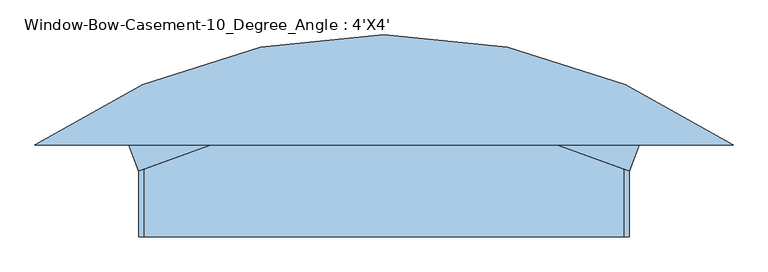
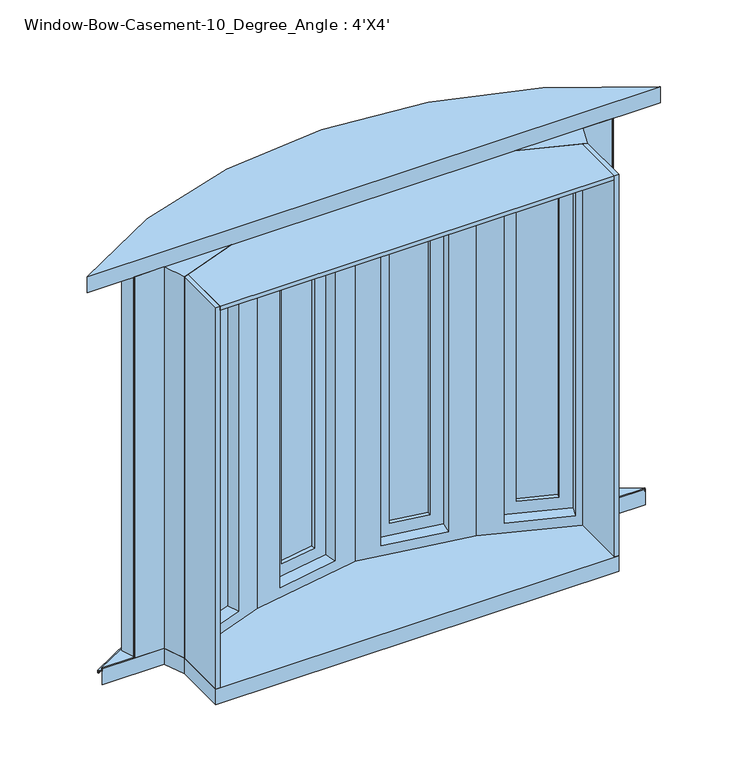
"""IFC4 building model written with IfcOpenShell, lengths in millimetres: window geometry, Window-Bow-Casement-10_Degree_Angle : 4'X4'."""

from ifc_helpers import new_model, si_unit, point, frame, frame_2d, origin, place, context, project, spatial, polyline, circle_curve, trimmed, segment, composite_curve, outline, extrude, faceted_brep, source, transform, mapped, element, save
from ifc_brep_helpers import plane_surface, cylinder_surface, revolved_surface, advanced_brep


def window_bow_casement_10_degree_angle_4_x4_fc1e5cf1(model_context):
    return source(origin(), model_context, "Body", "SolidModel", [
        advanced_brep(
        [(-820.9076978, 114.3, 663.1486341), (-820.9076978, 114.3, 660.4), (-728.4786409, 114.3, 660.4), (-728.4786409, 114.3, 663.1486341), (820.9076978, 114.3, 660.4), (820.9076978, 114.3, 663.1486341), (728.4786409, 114.3, 663.1486341), (728.4786409, 114.3, 660.4), (-820.9076978, 114.3, 653.0697935), (-821.7069058, 115.4458078, 663.1486341), (-821.7069058, 115.4458078, 654.4483503), (-828.9724329, 125.8622427, 652.2089977), (-828.9724329, 125.8622427, 643.2668038), (-826.7055885, 122.6123151, 643.2668038), (-826.7055885, 122.6123151, 644.7270038), (-828.0569765, 124.549772, 644.7270038), (-828.0569765, 124.549772, 650.8662705), (820.9076978, 114.3, 653.0697935), (828.0569765, 124.549772, 650.8662705), (828.0569765, 124.549772, 644.7270038), (826.7055885, 122.6123151, 644.7270038), (826.7055885, 122.6123151, 643.2668038), (828.9724329, 125.8622427, 643.2668038), (828.9724329, 125.8622427, 652.2089977), (821.7069058, 115.4458078, 654.4483503), (821.7069058, 115.4458078, 663.1486341)],
        [
            (0, 1),
            (1, 2),
            (2, 3),
            (3, 0),
            (4, 5),
            (5, 6),
            (6, 7),
            (7, 4),
            (8, 1),
            (0, 9),
            (9, 10),
            (10, 11),
            (11, 12),
            (12, 13),
            (13, 14),
            (14, 15),
            (15, 16),
            (16, 8),
            (17, 18),
            (18, 19),
            (19, 20),
            (20, 21),
            (21, 22),
            (22, 23),
            (23, 24),
            (24, 25),
            (25, 5),
            (4, 17),
            (8, 17, circle_curve(frame((0.0, -1062.6182794, 653.0697935), z_axis=(0.0, 0.0, -1.0), x_axis=(-0.5720887452257101, 0.8201917261141279, 0.0)), 1434.9306899)),
            (4, 1, circle_curve(frame((0.0, -1062.6182794, 660.4), z_axis=(0.0, 0.0, 1.0), x_axis=(-0.5720887452257101, 0.8201917261141279, 0.0)), 1434.9306899)),
            (7, 2, circle_curve(frame((0.0, -1062.6182794, 660.4), z_axis=(0.0, 0.0, 1.0), x_axis=(-0.5720887452257101, 0.8201917261141279, 0.0)), 1384.1306899)),
            (6, 3, circle_curve(frame((0.0, -1062.6182794, 663.1486341), z_axis=(0.0, 0.0, 1.0), x_axis=(-0.5720887452257101, 0.8201917261141279, 0.0)), 1384.1306899)),
            (25, 9, circle_curve(frame((0.0, -1062.6182794, 663.1486341), z_axis=(0.0, 0.0, 1.0), x_axis=(-0.5720887452257101, 0.8201917261141279, 0.0)), 1436.3276898)),
            (24, 10, circle_curve(frame((0.0, -1062.6182794, 654.4483503), z_axis=(0.0, 0.0, 1.0), x_axis=(-0.5720887452257101, 0.8201917261141279, 0.0)), 1436.3276898)),
            (23, 11, circle_curve(frame((0.0, -1062.6182794, 652.2089977), z_axis=(0.0, 0.0, 1.0), x_axis=(-0.5720887452257101, 0.8201917261141279, 0.0)), 1449.0276898)),
            (22, 12, circle_curve(frame((0.0, -1062.6182794, 643.2668038), z_axis=(0.0, 0.0, 1.0), x_axis=(-0.5720887452257101, 0.8201917261141279, 0.0)), 1449.0276898)),
            (21, 13, circle_curve(frame((0.0, -1062.6182794, 643.2668038), z_axis=(0.0, 0.0, 1.0), x_axis=(-0.5720887452257101, 0.8201917261141279, 0.0)), 1445.0652899)),
            (20, 14, circle_curve(frame((0.0, -1062.6182794, 644.7270038), z_axis=(0.0, 0.0, 1.0), x_axis=(-0.5720887452257101, 0.8201917261141279, 0.0)), 1445.0652899)),
            (19, 15, circle_curve(frame((0.0, -1062.6182794, 644.7270038), z_axis=(0.0, 0.0, 1.0), x_axis=(-0.5720887452257101, 0.8201917261141279, 0.0)), 1447.4274899)),
            (18, 16, circle_curve(frame((0.0, -1062.6182794, 650.8662705), z_axis=(0.0, 0.0, 1.0), x_axis=(-0.5720887452257101, 0.8201917261141279, 0.0)), 1447.4274899)),
        ],
        [
            plane_surface(frame((903.8545728, 114.3, 1270.0), z_axis=(0.0, -1.0, 0.0), x_axis=(0.0, 0.0, -1.0))),
            plane_surface(frame((-820.9076978, 114.3, 660.4), z_axis=(-0.8201917261141279, -0.5720887452257101, 0.0), x_axis=(0.0, 0.0, 1.0))),
            plane_surface(frame((820.9076978, 114.3, 660.4), z_axis=(0.8201917261141279, -0.5720887452257102, 0.0), x_axis=(0.0, 0.0, 1.0))),
            revolved_surface(polyline([(-820.9076978707535, 114.30000000321752, 653.0697935), (-820.9076978707535, 114.30000000321752, 660.4)]), (0.0, -1062.6182794, 660.4), (0.0, 0.0, -1.0)),
            plane_surface(frame((0.0, -1062.6182794, 660.4), z_axis=(0.0, 0.0, -1.0), x_axis=(-0.5720887452257101, 0.8201917261141279, 0.0))),
            revolved_surface(polyline([(-791.8455896132875, 72.63426031661993, 660.4), (-791.8455896132875, 72.63426031661993, 663.1486341)]), (0.0, -1062.6182794, 660.4), (0.0, 0.0, -1.0)),
            plane_surface(frame((0.0, -1062.6182794, 663.1486341), z_axis=(0.0, 0.0, 1.0), x_axis=(-0.5720887452257101, 0.8201917261141279, 0.0))),
            cylinder_surface(frame((0.0, -1062.6182794, 660.4), z_axis=(0.0, 0.0, -1.0), x_axis=(-0.5720887452257101, 0.8201917261141279, 0.0)), 1436.3276898),
            revolved_surface(polyline([(-821.7069058, 115.4458078, 654.4483503), (-828.9724329, 125.8622427, 652.2089977)]), (0.0, -1062.6182794, 660.4), (0.0, 0.0, -1.0)),
            cylinder_surface(frame((0.0, -1062.6182794, 660.4), z_axis=(0.0, 0.0, -1.0), x_axis=(-0.5720887452257101, 0.8201917261141279, 0.0)), 1449.0276898),
            plane_surface(frame((0.0, -1062.6182794, 643.2668038), z_axis=(0.0, 0.0, -1.0), x_axis=(-0.5720887452257101, 0.8201917261141279, 0.0))),
            revolved_surface(polyline([(-826.7055884681179, 122.61231507069374, 643.2668038), (-826.7055884681179, 122.61231507069374, 644.7270038)]), (0.0, -1062.6182794, 660.4), (0.0, 0.0, -1.0)),
            plane_surface(frame((0.0, -1062.6182794, 644.7270038), z_axis=(0.0, 0.0, 1.0), x_axis=(-0.5720887452257101, 0.8201917261141279, 0.0))),
            revolved_surface(polyline([(-828.0569765020902, 124.54977196612049, 644.7270038), (-828.0569765020902, 124.54977196612049, 650.8662705)]), (0.0, -1062.6182794, 660.4), (0.0, 0.0, -1.0)),
            revolved_surface(polyline([(-828.0569765, 124.549772, 650.8662705), (-820.9076978, 114.3, 653.0697935)]), (0.0, -1062.6182794, 660.4), (0.0, 0.0, -1.0)),
        ],
        [
            (0, [[1, 2, 3, 4]]),
            (0, [[5, 6, 7, 8]]),
            (1, [[9, -1, 10, 11, 12, 13, 14, 15, 16, 17, 18]]),
            (2, [[19, 20, 21, 22, 23, 24, 25, 26, 27, -5, 28]]),
            (3, [[-9, 29, -28, 30]]),
            (4, [[-30, -8, 31, -2]]),
            (5, [[-31, -7, 32, -3]]),
            (6, [[33, -10, -4, -32, -6, -27]]),
            (7, [[-11, -33, -26, 34]]),
            (8, [[-12, -34, -25, 35]]),
            (9, [[-13, -35, -24, 36]]),
            (10, [[-14, -36, -23, 37]]),
            (11, [[-15, -37, -22, 38]]),
            (12, [[-16, -38, -21, 39]]),
            (13, [[-17, -39, -20, 40]]),
            (14, [[-18, -40, -19, -29]]),
        ],
    ),
        extrude(outline(polyline([(-692.8458946, 125.1591396), (-722.6811353, 114.3), (-737.8839307, 156.069337), (-708.04869, 166.9284765), (-692.8458946, 125.1591396)])), frame((0.0, 0.0, 663.1486341), z_axis=(0.0, 0.0, 1.0), x_axis=(1.0, 0.0, 0.0)), (0.0, 0.0, 1.0), 1216.4513659),
        extrude(outline(polyline([(692.8458946, 125.1591396), (708.04869, 166.9284765), (737.8839307, 156.069337), (722.6811353, 114.3), (692.8458946, 125.1591396)])), frame((0.0, 0.0, 663.1486341), z_axis=(0.0, 0.0, 1.0), x_axis=(1.0, 0.0, 0.0)), (0.0, 0.0, 1.0), 1216.4513659),
        faceted_brep([(0.0, 208.5319163, 1879.6), (330.4505105, 150.2645755, 1879.6), (356.846972, 248.7775109, 1879.6), (0.0, 311.6992601, 1879.6), (280.5494558, 197.7512317, 1866.9), (57.0219627, 237.1651597, 1866.9), (68.048622, 299.700452, 1866.9), (291.5761151, 260.2865241, 1866.9), (255.1728726, 163.5380541, 1847.85), (69.1665548, 196.3359865, 1847.85), (75.7825504, 233.8571619, 1847.85), (261.7888681, 201.0592295, 1847.85), (57.0219627, 237.1651597, 673.1), (68.048622, 299.700452, 673.1), (69.1665548, 196.3359865, 692.15), (75.7825504, 233.8571619, 692.15), (0.0, 311.6992601, 660.4), (356.846972, 248.7775109, 660.4), (330.4505105, 150.2645755, 660.4), (0.0, 208.5319163, 660.4), (280.5494558, 197.7512317, 673.1), (291.5761151, 260.2865241, 673.1), (255.1728726, 163.5380541, 692.15), (261.7888681, 201.0592295, 692.15)], [[[0, 1, 2, 3]], [[4, 5, 6, 7]], [[8, 9, 10, 11]], [[5, 12, 13, 6]], [[9, 14, 15, 10]], [[16, 17, 18, 19]], [[12, 20, 21, 13]], [[14, 22, 23, 15]], [[2, 17, 16, 3], [6, 13, 21, 7]], [[7, 21, 20, 4]], [[4, 20, 12, 5], [10, 15, 23, 11]], [[11, 23, 22, 8]], [[18, 1, 0, 19], [8, 22, 14, 9]], [[3, 16, 19, 0]], [[1, 18, 17, 2]]]),
        extrude(outline(polyline([(229.7810224, 238.9428712), (228.6783565, 232.689342), (117.7143895, 252.2552833), (118.8170554, 258.5088125), (229.7810224, 238.9428712)])), frame((0.0, 0.0, 730.25), z_axis=(0.0, 0.0, 1.0), x_axis=(1.0, 0.0, 0.0)), (0.0, 0.0, 1.0), 1079.5),
        extrude(outline(polyline([(227.5756905, 226.4358128), (226.4730246, 220.1822836), (115.5090576, 239.7482248), (116.6117235, 246.0017541), (227.5756905, 226.4358128)])), frame((0.0, 0.0, 730.25), z_axis=(0.0, 0.0, 1.0), x_axis=(1.0, 0.0, 0.0)), (0.0, 0.0, 1.0), 1079.5),
        extrude(outline(polyline([(1136.65, 57.1499999), (1136.65, -169.8257651), (-57.15, -169.8257651), (-57.15, 57.1499999), (1136.65, 57.1499999)]), holes=[polyline([(1079.5, -112.6757651), (1079.5, 0.0), (0.0, 0.0), (0.0, -112.6757651), (1079.5, -112.6757651)])]), frame((224.2676928, 207.6752251, 730.25), z_axis=(0.17364817766693014, 0.9848077530122081, 0.0), x_axis=(0.0, 0.0, 1.0)), (0.0, 0.0, 1.0), 44.45),
        faceted_brep([(0.0, 208.5319163, 1879.6), (0.0, 311.6992601, 1879.6), (-356.846972, 248.7775109, 1879.6), (-330.4505105, 150.2645755, 1879.6), (-280.5494558, 197.7512317, 1866.9), (-291.5761151, 260.2865241, 1866.9), (-68.048622, 299.700452, 1866.9), (-57.0219627, 237.1651597, 1866.9), (-255.1728726, 163.5380541, 1847.85), (-261.7888681, 201.0592295, 1847.85), (-75.7825504, 233.8571619, 1847.85), (-69.1665548, 196.3359865, 1847.85), (-68.048622, 299.700452, 673.1), (-57.0219627, 237.1651597, 673.1), (-75.7825504, 233.8571619, 692.15), (-69.1665548, 196.3359865, 692.15), (0.0, 311.6992601, 660.4), (0.0, 208.5319163, 660.4), (-330.4505105, 150.2645755, 660.4), (-356.846972, 248.7775109, 660.4), (-291.5761151, 260.2865241, 673.1), (-280.5494558, 197.7512317, 673.1), (-261.7888681, 201.0592295, 692.15), (-255.1728726, 163.5380541, 692.15)], [[[0, 1, 2, 3]], [[4, 5, 6, 7]], [[8, 9, 10, 11]], [[7, 6, 12, 13]], [[11, 10, 14, 15]], [[16, 17, 18, 19]], [[13, 12, 20, 21]], [[15, 14, 22, 23]], [[2, 1, 16, 19], [6, 5, 20, 12]], [[5, 4, 21, 20]], [[4, 7, 13, 21], [10, 9, 22, 14]], [[9, 8, 23, 22]], [[18, 17, 0, 3], [8, 11, 15, 23]], [[1, 0, 17, 16]], [[3, 2, 19, 18]]]),
        extrude(outline(polyline([(-229.7810224, 238.9428712), (-118.8170554, 258.5088125), (-117.7143895, 252.2552833), (-228.6783565, 232.689342), (-229.7810224, 238.9428712)])), frame((0.0, 0.0, 730.25), z_axis=(0.0, 0.0, 1.0), x_axis=(1.0, 0.0, 0.0)), (0.0, 0.0, 1.0), 1079.5),
        extrude(outline(polyline([(-227.5756905, 226.4358128), (-116.6117235, 246.0017541), (-115.5090576, 239.7482248), (-226.4730246, 220.1822836), (-227.5756905, 226.4358128)])), frame((0.0, 0.0, 730.25), z_axis=(0.0, 0.0, 1.0), x_axis=(1.0, 0.0, 0.0)), (0.0, 0.0, 1.0), 1079.5),
        extrude(outline(polyline([(1136.65, -57.1499999), (-57.15, -57.1499999), (-57.15, 169.8257651), (1136.65, 169.8257651), (1136.65, -57.1499999)]), holes=[polyline([(1079.5, 112.6757651), (0.0, 112.6757651), (0.0, 0.0), (1079.5, 0.0), (1079.5, 112.6757651)])]), frame((-224.2676928, 207.6752251, 730.25), z_axis=(-0.17364817766693014, 0.9848077530122081, 0.0), x_axis=(0.0, 0.0, 1.0)), (0.0, 0.0, 1.0), 44.45),
        faceted_brep([(330.4505105, 150.2645755, 1879.6), (609.6, 48.6624704, 1879.6), (633.490107, 114.3, 1879.6), (726.3208967, 114.3, 1879.6), (356.846972, 248.7775109, 1879.6), (610.6968712, 88.8084151, 1866.9), (397.4094197, 166.4386988, 1866.9), (419.1276988, 226.1091802, 1866.9), (632.4151503, 148.4788965, 1866.9), (579.7647593, 59.52161, 1847.85), (402.2795966, 124.1209262, 1847.85), (415.3105641, 159.9232151, 1847.85), (592.7957267, 95.3238988, 1847.85), (397.4094197, 166.4386988, 673.1), (419.1276988, 226.1091802, 673.1), (402.2795966, 124.1209262, 692.15), (415.3105641, 159.9232151, 692.15), (356.846972, 248.7775109, 660.4), (726.3208967, 114.3, 660.4), (633.490107, 114.3, 660.4), (609.6, 48.6624704, 660.4), (330.4505105, 150.2645755, 660.4), (610.6968712, 88.8084151, 673.1), (632.4151503, 148.4788965, 673.1), (579.7647593, 59.52161, 692.15), (592.7957267, 95.3238988, 692.15)], [[[0, 1, 2, 3, 4]], [[5, 6, 7, 8]], [[9, 10, 11, 12]], [[6, 13, 14, 7]], [[10, 15, 16, 11]], [[17, 18, 19, 20, 21]], [[13, 22, 23, 14]], [[15, 24, 25, 16]], [[20, 19, 2, 1]], [[3, 18, 17, 4], [7, 14, 23, 8]], [[8, 23, 22, 5]], [[5, 22, 13, 6], [11, 16, 25, 12]], [[12, 25, 24, 9]], [[1, 0, 21, 20], [9, 24, 15, 10]], [[2, 19, 18, 3]], [[4, 17, 21, 0]]]),
        extrude(outline(polyline([(567.8525774, 138.190107), (565.6807495, 132.2230589), (459.8001646, 170.7604402), (461.9719925, 176.7274883), (567.8525774, 138.190107)])), frame((0.0, 0.0, 730.25), z_axis=(0.0, 0.0, 1.0), x_axis=(1.0, 0.0, 0.0)), (0.0, 0.0, 1.0), 1079.5),
        extrude(outline(polyline([(563.5089216, 126.2560107), (561.3370937, 120.2889626), (455.4565088, 158.8263439), (457.6283367, 164.793392), (563.5089216, 126.2560107)])), frame((0.0, 0.0, 730.25), z_axis=(0.0, 0.0, 1.0), x_axis=(1.0, 0.0, 0.0)), (0.0, 0.0, 1.0), 1079.5),
        extrude(outline(polyline([(1136.65, 57.15), (1136.65, -169.825765), (-57.15, -169.825765), (-57.15, 57.15), (1136.65, 57.15)]), holes=[polyline([(1079.5, -112.6757651), (1079.5, 0.0), (0.0, 0.0), (0.0, -112.6757651), (1079.5, -112.6757651)])]), frame((556.9934379, 108.3548663, 730.25), z_axis=(0.3420201433256678, 0.9396926207859088, 0.0), x_axis=(0.0, 0.0, 1.0)), (0.0, 0.0, 1.0), 44.45),
        faceted_brep([(-330.4505105, 150.2645755, 1879.6), (-356.846972, 248.7775109, 1879.6), (-726.3208967, 114.3, 1879.6), (-633.490107, 114.3, 1879.6), (-609.6, 48.6624704, 1879.6), (-610.6968712, 88.8084151, 1866.9), (-632.4151503, 148.4788965, 1866.9), (-419.1276988, 226.1091802, 1866.9), (-397.4094197, 166.4386988, 1866.9), (-579.7647593, 59.52161, 1847.85), (-592.7957267, 95.3238988, 1847.85), (-415.3105641, 159.9232151, 1847.85), (-402.2795966, 124.1209262, 1847.85), (-419.1276988, 226.1091802, 673.1), (-397.4094197, 166.4386988, 673.1), (-415.3105641, 159.9232151, 692.15), (-402.2795966, 124.1209262, 692.15), (-356.846972, 248.7775109, 660.4), (-330.4505105, 150.2645755, 660.4), (-609.6, 48.6624704, 660.4), (-633.490107, 114.3, 660.4), (-726.3208967, 114.3, 660.4), (-632.4151503, 148.4788965, 673.1), (-610.6968712, 88.8084151, 673.1), (-592.7957267, 95.3238988, 692.15), (-579.7647593, 59.52161, 692.15)], [[[0, 1, 2, 3, 4]], [[5, 6, 7, 8]], [[9, 10, 11, 12]], [[8, 7, 13, 14]], [[12, 11, 15, 16]], [[17, 18, 19, 20, 21]], [[14, 13, 22, 23]], [[16, 15, 24, 25]], [[19, 4, 3, 20]], [[2, 1, 17, 21], [7, 6, 22, 13]], [[6, 5, 23, 22]], [[5, 8, 14, 23], [11, 10, 24, 15]], [[10, 9, 25, 24]], [[4, 19, 18, 0], [9, 12, 16, 25]], [[3, 2, 21, 20]], [[1, 0, 18, 17]]]),
        extrude(outline(polyline([(-567.8525774, 138.190107), (-461.9719925, 176.7274883), (-459.8001646, 170.7604402), (-565.6807495, 132.2230589), (-567.8525774, 138.190107)])), frame((0.0, 0.0, 730.25), z_axis=(0.0, 0.0, 1.0), x_axis=(1.0, 0.0, 0.0)), (0.0, 0.0, 1.0), 1079.5),
        extrude(outline(polyline([(-563.5089216, 126.2560107), (-457.6283367, 164.793392), (-455.4565088, 158.8263439), (-561.3370937, 120.2889626), (-563.5089216, 126.2560107)])), frame((0.0, 0.0, 730.25), z_axis=(0.0, 0.0, 1.0), x_axis=(1.0, 0.0, 0.0)), (0.0, 0.0, 1.0), 1079.5),
        extrude(outline(polyline([(1136.65, -57.15), (-57.15, -57.15), (-57.15, 169.825765), (1136.65, 169.825765), (1136.65, -57.15)]), holes=[polyline([(1079.5, 112.6757651), (0.0, 112.6757651), (0.0, 0.0), (1079.5, 0.0), (1079.5, 112.6757651)])]), frame((-556.9934379, 108.3548663, 730.25), z_axis=(-0.3420201433256678, 0.9396926207859088, 0.0), x_axis=(0.0, 0.0, 1.0)), (0.0, 0.0, 1.0), 44.45),
        extrude(outline(composite_curve([segment(trimmed(circle_curve(frame_2d((0.0, -1123.2314298)), 1511.1306899), [point((-867.1977411, 114.3))], [point((867.1977411, 114.3))], False, "CARTESIAN"), True, "CONTINUOUS"), segment(polyline([(867.1977411, 114.3), (-867.1977411, 114.3)]), True, "CONTINUOUS")], self_intersect=False)), frame((0.0, 0.0, 1879.6), z_axis=(0.0, 0.0, 1.0), x_axis=(1.0, 0.0, 0.0)), (0.0, 0.0, 1.0), 50.8),
        extrude(outline(polyline([(-609.6, -114.3), (-609.6, 48.6624704), (-596.9, 53.2848924), (-596.9, -114.3), (-609.6, -114.3)])), frame((0.0, 0.0, 660.4), z_axis=(0.0, 0.0, 1.0), x_axis=(1.0, 0.0, 0.0)), (0.0, 0.0, 1.0), 1219.2),
        extrude(outline(polyline([(609.6, -114.3), (596.9, -114.3), (596.9, 53.2848924), (609.6, 48.6624704), (609.6, -114.3)])), frame((0.0, 0.0, 660.4), z_axis=(0.0, 0.0, 1.0), x_axis=(1.0, 0.0, 0.0)), (0.0, 0.0, 1.0), 1219.2),
        extrude(outline(polyline([(-330.4505105, 150.2645755), (0.0, 208.5319163), (330.4505105, 150.2645755), (596.9, 53.2848924), (596.9, -114.3), (-596.9, -114.3), (-596.9, 53.2848924), (-330.4505105, 150.2645755)])), frame((0.0, 0.0, 1866.9), z_axis=(0.0, 0.0, 1.0), x_axis=(1.0, 0.0, 0.0)), (0.0, 0.0, 1.0), 12.7),
        extrude(outline(composite_curve([segment(trimmed(circle_curve(frame_2d((0.0, -1123.2314298)), 1485.7306899), [point((-822.1384574, 114.3))], [point((822.1384574, 114.3))], False, "CARTESIAN"), True, "CONTINUOUS"), segment(polyline([(822.1384574, 114.3), (633.490107, 114.3), (609.6, 48.6624704), (609.6, -114.3), (-609.6, -114.3), (-609.6, 48.6624704), (-633.490107, 114.3), (-822.1384574, 114.3)]), True, "CONTINUOUS")], self_intersect=False)), frame((0.0, 0.0, 609.6), z_axis=(0.0, 0.0, 1.0), x_axis=(1.0, 0.0, 0.0)), (0.0, 0.0, 1.0), 50.8),
    ])


if __name__ == "__main__":
    model = new_model("IFC4")
    model_context = context("Model", 3, world=origin())
    ifc_project = project(units=[si_unit("LENGTHUNIT", "METRE", prefix="MILLI")], contexts=[model_context])
    site = spatial("IfcSite", under=ifc_project)
    building = spatial("IfcBuilding", under=site)
    placement = place(None, origin())
    window_bow_casement_10_degree_angle_4_x4_shape = window_bow_casement_10_degree_angle_4_x4_fc1e5cf1(model_context)
    element("IfcWindow", 1, ObjectType="Window-Bow-Casement-10_Degree_Angle : 4'X4'", at=placement, inside=building, context=model_context, shape_type="MappedRepresentation", body=[
        mapped(window_bow_casement_10_degree_angle_4_x4_shape, transform((0.0, 0.0, 0.0), x_axis=(1.0, 0.0, 0.0), y_axis=(0.0, 1.0, 0.0), z_axis=(0.0, 0.0, 1.0))),
    ])
    save(model, "model.ifc")

# Revit data of these elements
# Type "Window-Bow-Casement-10_Degree_Angle : 4'X4'"
#   Type Mark = "27"
#   Fire Rating = "0.5h"
#   Assembly Code = "B2020100"
#   Analytic Construction = "Double glazing - domestic"
#   Width = 4' - 0"
#   Visual Light Transmittance = 0.81
#   Thermal Resistance (R) = 1.8146 (h·ft²·°F)/BTU
#   Solar Heat Gain Coefficient = 0.76
#   Rough Width = 4' - 0 1/2"
#   Rough Height = 4' - 0 1/2"
#   Radius 3 = 4' - 11.49333"
#   Radius 2 = 4' - 10.49333"
#   Radius 1 = 4' - 8.49333"
#   Length 7 = 4' - 9.19062"
#   Length 6 = 0' - 1.41593"
#   Length 5 = 1' - 1.00986"
#   Length 2 = 0' - 2.58415"
#   Depth 2 = 0' - 6.3557"
#   Length 4 = 0' - 1.03923"
#   Length 3 = 0' - 0.32476"
#   Length 1 = 0' - 10.27567"
#   Wall Thickness [instance default] = 0' - 6"
#   Trim Width = 4' - 4.64952"
#   Trim Height = 4' - 0"
#   Height 1 = 4' - 2"
#   Height = 4' - 0"
#   Heat Transfer Coefficient (U) = 0.5511 BTU/(h·ft²·°F)
#   Depth 1 = 0' - 5.29439"
#   Default Sill Height = 2' - 0"
#   Angle 2 = 15.00°
#   Angle 1 = 10.00°
#   Angle = 20.00°
#   Muntin Visibility = yes
#   Interior Trim Visibility [instance default] = yes
#   Exterior Trim Visibility [instance default] = yes
#   Muntin Pattern = Muntin Pattern_2x2 : Muntin Pattern_2x2
#   Interior Trim Material = Wood - Stained
#   Exterior Trim Material = Clad - White
#   Interior Trim = Trim-Window-Interior-Flat : Picture Frame
#   Interior Frame Material = Wood - Stained
#   Glass Panel Material = Glass
#   Exterior Frame Material = Clad - White
#   Wall Closure = (empty or 0)
# Element 1 (IfcWindow, "Window-Bow-Casement-10_Degree_Angle : 4'X4'")
#   Wall Thickness = 0' - 9"
#   Materials on its faces: "Wood - Stained", "Clad - White", "Glass"
# Materials
#   "Wood - Stained": class "Wood", colour RGB 224 178 126, transparency 0, Cost = 0
#   "Clad - White": class "Wood", colour RGB 242 242 238, transparency 0, Cost = 0
#   "Glass": class "Glass", colour RGB 0 128 192, transparency 0.75, Description = "Soda Lime Glass", Cost = 0
